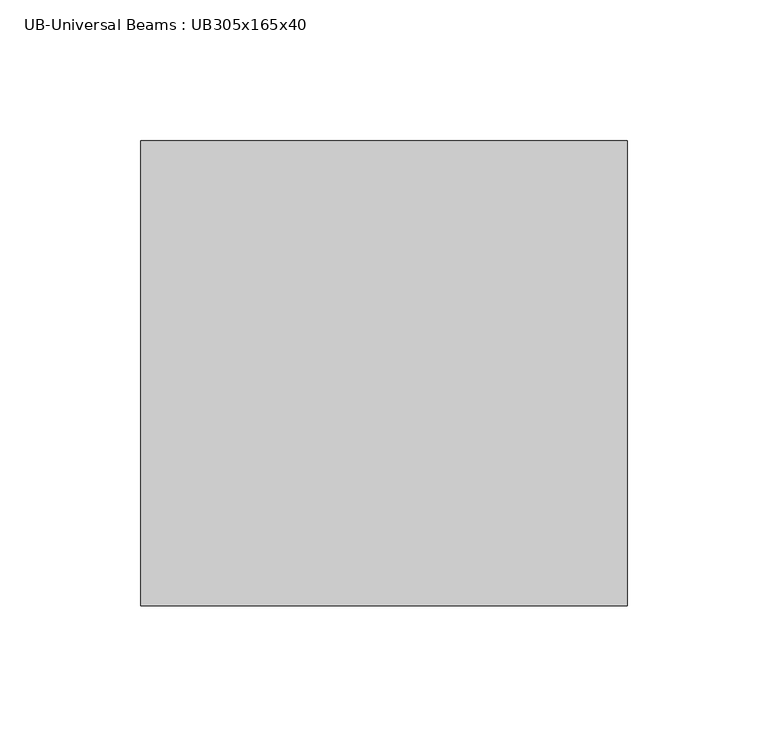
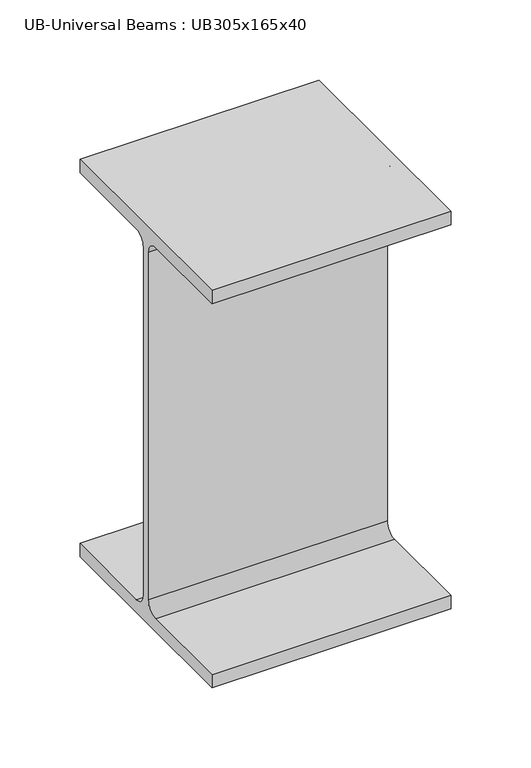
"""IFC4 building model written with IfcOpenShell, lengths in millimetres: beam geometry, UB-Universal Beams : UB305x165x40."""

from ifc_helpers import new_model, si_unit, point, frame, frame_2d, origin, place, context, project, spatial, polyline, circle_curve, trimmed, segment, composite_curve, outline, extrude, source, transform, mapped, element, save


def ub_universal_beams_ub305x165x40_7a055ae5(model_context):
    return source(origin(), model_context, "Body", "SweptSolid", [
        extrude(outline(composite_curve([segment(polyline([(82.5, -141.5), (82.5, -151.7), (-82.5, -151.7), (-82.5, -141.5), (-11.9, -141.5)]), True, "CONTINUOUS"), segment(trimmed(circle_curve(frame_2d((-11.9, -132.6)), 8.9), [point((-11.9, -141.5))], [point((-3.0, -132.6))], True, "CARTESIAN"), True, "CONTINUOUS"), segment(polyline([(-3.0, -132.6), (-3.0, 132.6)]), True, "CONTINUOUS"), segment(trimmed(circle_curve(frame_2d((-11.9, 132.6)), 8.9), [point((-3.0, 132.6))], [point((-11.9, 141.5))], True, "CARTESIAN"), True, "CONTINUOUS"), segment(polyline([(-11.9, 141.5), (-82.5, 141.5), (-82.5, 151.7), (82.5, 151.7), (82.5, 141.5), (11.9, 141.5)]), True, "CONTINUOUS"), segment(trimmed(circle_curve(frame_2d((11.9, 132.6)), 8.9), [point((11.9, 141.5))], [point((3.0, 132.6))], True, "CARTESIAN"), True, "CONTINUOUS"), segment(polyline([(3.0, 132.6), (3.0, -132.6)]), True, "CONTINUOUS"), segment(trimmed(circle_curve(frame_2d((11.9, -132.6)), 8.9), [point((3.0, -132.6))], [point((11.9, -141.5))], True, "CARTESIAN"), True, "CONTINUOUS"), segment(polyline([(11.9, -141.5), (82.5, -141.5)]), True, "CONTINUOUS")], self_intersect=False)), frame((-60.85, 0.0, 0.0), z_axis=(1.0, 0.0, 0.0), x_axis=(0.0, 1.0, 0.0)), (0.0, 0.0, 1.0), 172.6),
    ])


if __name__ == "__main__":
    model = new_model("IFC4")
    model_context = context("Model", 3, world=origin())
    ifc_project = project(units=[si_unit("LENGTHUNIT", "METRE", prefix="MILLI")], contexts=[model_context])
    site = spatial("IfcSite", under=ifc_project)
    building = spatial("IfcBuilding", under=site)
    placement = place(None, origin())
    ub_universal_beams_ub305x165x40_shape = ub_universal_beams_ub305x165x40_7a055ae5(model_context)
    element("IfcBeam", 1, ObjectType="UB-Universal Beams : UB305x165x40", at=placement, inside=building, context=model_context, shape_type="MappedRepresentation", body=[
        mapped(ub_universal_beams_ub305x165x40_shape, transform((0.0, 0.0, 0.0), x_axis=(1.0, 0.0, 0.0), y_axis=(0.0, 1.0, 0.0), z_axis=(0.0, 0.0, 1.0))),
    ])
    save(model, "model.ifc")

# Revit data of these elements
# Type "UB-Universal Beams : UB305x165x40"
#   Section Name Key = "UB305X165X40"
#   Width = 16.5 cm
#   Web Thickness = 0.6 cm
#   Web Fillet = 0.89 cm
#   Warping Constant = 164000.0 cm⁶
#   Torsional Moment of Inertia = 14.70 cm⁴
#   Section Area = 51.3 cm²
#   Plastic Modulus weak axis = 142.0 cm³
#   Plastic Modulus strong axis = 623.0 cm³
#   Nominal Weight = 40.2999 kgf/m
#   Moment of Inertia weak axis = 764.00 cm⁴
#   Moment of Inertia strong axis = 8503.00 cm⁴
#   Height = 30.34 cm
#   Flange Thickness = 1.02 cm
#   Elastic Modulus weak axis = 92.6 cm³
#   Elastic Modulus strong axis = 560.0 cm³
#   Centroid Vertical = 15.17 cm
#   Centroid Horizontal = 8.25 cm
#   Bolt Spacing = 9.0 cm
#   Length [instance default] = 1500 mm
#   Structural Material [instance default] = Metal - Steel 43-275
#   Type Comments = ""
#   Assembly Code = ""
# Element 1 (IfcBeam, "UB-Universal Beams : UB305x165x40")
#   Materials on its faces: "Metal - Steel 43-275"
# Materials
#   "Metal - Steel 43-275": class "Metal", colour RGB 247 247 247, transparency 0, Cost = 0
